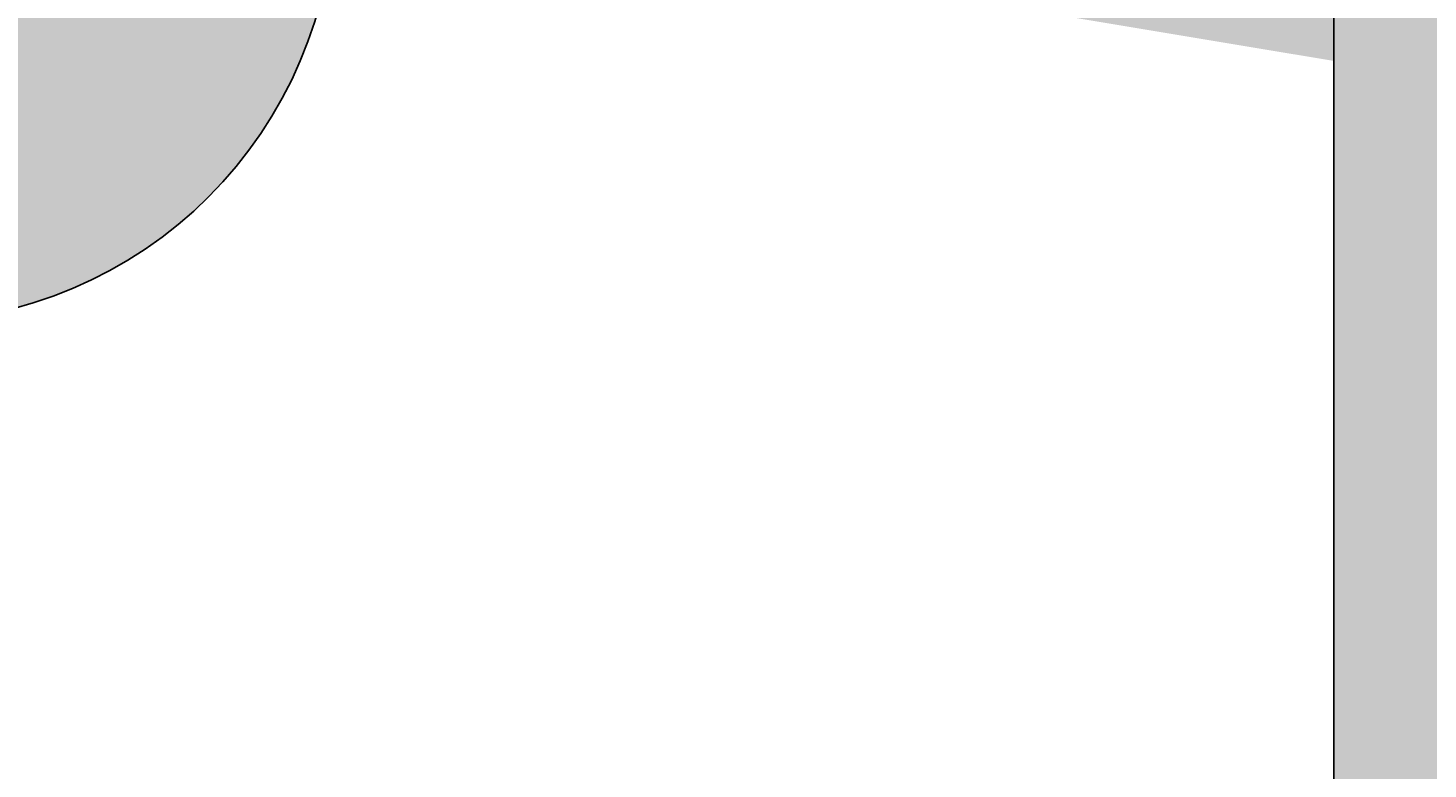
# Model space of a CAD drawing. Units: millimetres. Extents: x -22994 to 29398, y -19990 to 20176.
# Tile 18 of 135: x 54 to 99, y 52 to 76. Entities that reach past the tile are written whole.
import ezdxf

# ---------------------------------------------------------------- set-up
doc = ezdxf.new("R2010")
doc.units = ezdxf.units.MM
doc.header["$MEASUREMENT"] = 0
for name, color, linetype, lineweight in [('M-DIMS', 2, 'Continuous', 18), ('M-EQPM', 7, 'Continuous', 25), ('M-EQPM-PATT', 7, 'Continuous', 18)]:
    doc.layers.add(name, color=color, linetype=linetype, lineweight=lineweight)
doc.styles.get("Standard").update_dxf_attribs({"font": 'arial.ttf'})
doc.dimstyles.get("Standard").update_dxf_attribs({"dimtxt": 0.18, "dimasz": 10000, "dimexe": 0.18, "dimexo": 0.0625, "dimgap": 0.09, "dimtad": 0, "dimtih": 1, "dimtoh": 1, "dimdec": 0, "dimzin": 0, "dimdsep": 46, "dimtxsty": 'Standard', "dimcen": 0.09, "dimadec": 0, "dimazin": 0, "dimtfac": 1, "dimtdec": 0, "dimtofl": 0, "dimtmove": 0, "dimatfit": 3, "dimfxl": 1, "dimtolj": 1, "dimtzin": 0, "dimlwd": 30, "dimarcsym": 0})

# ---------------------------------------------------------------- blocks, each defined once
blk = doc.blocks.new('*D2')
at = {"layer": 'Defpoints', "color": 0, "transparency": 16777216}
for p in [(6.677, 10.271), (290.852, 10.271), (290.852, -5.079)]:
    blk.add_point(p, dxfattribs=at)
at = {"layer": 'M-DIMS', "color": 0, "lineweight": -2, "transparency": 16777216}
for p, q in [((6.677, 10.209), (6.677, -5.259)), ((290.852, 10.209), (290.852, -5.259))]:
    blk.add_line(p, q, dxfattribs=at)
at = {"layer": 'M-DIMS', "color": 0, "lineweight": 30, "transparency": 16777216}
for p, q in [((-9993.323, -5.079), (-19993.323, -5.079)), ((10290.852, -5.079), (20290.852, -5.079))]:
    blk.add_line(p, q, dxfattribs=at)
at = {"layer": 'M-DIMS', "color": 0, "transparency": 16777216}
for points in [[(-9993.323, 1661.588), (-9993.323, -1671.745), (6.677, -5.079)], [(10290.852, 1661.588), (10290.852, -1671.745), (290.852, -5.079)]]:
    blk.add_solid(points, dxfattribs=at)
at = {"layer": 'M-DIMS', "color": 0, "transparency": 16777216, "insert": (148.765, -5.079), "char_height": 0.18, "attachment_point": 5}
blk.add_mtext('\\A1;284.2', dxfattribs=at)
blk = doc.blocks.new('*D3')
at = {"layer": 'Defpoints', "color": 0, "transparency": 16777216}
for p in [(110.265, 204.165), (110.265, 176.366), (95.833, 127.967)]:
    blk.add_point(p, dxfattribs=at)
at = {"layer": 'M-DIMS', "color": 0, "lineweight": 30, "transparency": 16777216}
for p, q in [((-9904.167, 204.165), (-19904.167, 204.165)), ((10110.265, 204.165), (20110.265, 204.165))]:
    blk.add_line(p, q, dxfattribs=at)
at = {"layer": 'M-DIMS', "color": 0, "lineweight": -2, "transparency": 16777216}
for p, q in [((95.833, 128.03), (95.833, 204.345)), ((110.265, 176.429), (110.265, 204.345))]:
    blk.add_line(p, q, dxfattribs=at)
at = {"layer": 'M-DIMS', "color": 0, "transparency": 16777216}
for points in [[(-9904.167, 1870.832), (-9904.167, -1462.501), (95.833, 204.165)], [(10110.265, 1870.832), (10110.265, -1462.501), (110.265, 204.165)]]:
    blk.add_solid(points, dxfattribs=at)
at = {"layer": 'M-DIMS', "color": 0, "transparency": 16777216, "insert": (103.049, 204.165), "char_height": 0.18, "attachment_point": 5}
blk.add_mtext('\\A1;14.432', dxfattribs=at)
blk = doc.blocks.new('*D4')
at = {"layer": 'Defpoints', "color": 0, "transparency": 16777216}
for p in [(116.265, 204.165), (110.265, 176.366), (116.265, 176.366)]:
    blk.add_point(p, dxfattribs=at)
at = {"layer": 'M-DIMS', "color": 0, "lineweight": 30, "transparency": 16777216}
for p, q in [((-9889.735, 204.165), (-19889.735, 204.165)), ((10116.265, 204.165), (20116.265, 204.165))]:
    blk.add_line(p, q, dxfattribs=at)
at = {"layer": 'M-DIMS', "color": 0, "lineweight": -2, "transparency": 16777216}
for p, q in [((110.265, 176.429), (110.265, 204.345)), ((116.265, 176.429), (116.265, 204.345))]:
    blk.add_line(p, q, dxfattribs=at)
at = {"layer": 'M-DIMS', "color": 0, "transparency": 16777216}
for points in [[(-9889.735, 1870.832), (-9889.735, -1462.501), (110.265, 204.165)], [(10116.265, 1870.832), (10116.265, -1462.501), (116.265, 204.165)]]:
    blk.add_solid(points, dxfattribs=at)
at = {"layer": 'M-DIMS', "color": 0, "transparency": 16777216, "insert": (113.265, 204.165), "char_height": 0.18, "attachment_point": 5}
blk.add_mtext('\\A1;6', dxfattribs=at)
blk = doc.blocks.new('*D5')
at = {"layer": 'Defpoints', "color": 0, "transparency": 16777216}
for p in [(181.265, 204.165), (116.265, 176.366), (181.265, 176.366)]:
    blk.add_point(p, dxfattribs=at)
at = {"layer": 'M-DIMS', "color": 0, "lineweight": 30, "transparency": 16777216}
for p, q in [((-9883.735, 204.165), (-19883.735, 204.165)), ((10181.265, 204.165), (20181.265, 204.165))]:
    blk.add_line(p, q, dxfattribs=at)
at = {"layer": 'M-DIMS', "color": 0, "lineweight": -2, "transparency": 16777216}
for p, q in [((116.265, 176.429), (116.265, 204.345)), ((181.265, 176.429), (181.265, 204.345))]:
    blk.add_line(p, q, dxfattribs=at)
at = {"layer": 'M-DIMS', "color": 0, "transparency": 16777216}
for points in [[(-9883.735, 1870.832), (-9883.735, -1462.501), (116.265, 204.165)], [(10181.265, 1870.832), (10181.265, -1462.501), (181.265, 204.165)]]:
    blk.add_solid(points, dxfattribs=at)
at = {"layer": 'M-DIMS', "color": 0, "transparency": 16777216, "insert": (148.765, 204.165), "char_height": 0.18, "attachment_point": 5}
blk.add_mtext('\\A1;65', dxfattribs=at)
blk = doc.blocks.new('*D6')
at = {"layer": 'Defpoints', "color": 0, "transparency": 16777216}
for p in [(187.265, 204.165), (181.265, 176.366), (187.265, 176.366)]:
    blk.add_point(p, dxfattribs=at)
at = {"layer": 'M-DIMS', "color": 0, "lineweight": 30, "transparency": 16777216}
for p, q in [((-9818.735, 204.165), (-19818.735, 204.165)), ((10187.265, 204.165), (20187.265, 204.165))]:
    blk.add_line(p, q, dxfattribs=at)
at = {"layer": 'M-DIMS', "color": 0, "lineweight": -2, "transparency": 16777216}
for p, q in [((181.265, 176.429), (181.265, 204.345)), ((187.265, 176.429), (187.265, 204.345))]:
    blk.add_line(p, q, dxfattribs=at)
at = {"layer": 'M-DIMS', "color": 0, "transparency": 16777216}
for points in [[(-9818.735, 1870.832), (-9818.735, -1462.501), (181.265, 204.165)], [(10187.265, 1870.832), (10187.265, -1462.501), (187.265, 204.165)]]:
    blk.add_solid(points, dxfattribs=at)
at = {"layer": 'M-DIMS', "color": 0, "transparency": 16777216, "insert": (184.265, 204.165), "char_height": 0.18, "attachment_point": 5}
blk.add_mtext('\\A1;6', dxfattribs=at)
blk = doc.blocks.new('*D7')
at = {"layer": 'Defpoints', "color": 0, "transparency": 16777216}
for p in [(201.697, 204.165), (187.265, 176.366), (201.697, 127.967)]:
    blk.add_point(p, dxfattribs=at)
at = {"layer": 'M-DIMS', "color": 0, "lineweight": 30, "transparency": 16777216}
for p, q in [((-9812.735, 204.165), (-19812.735, 204.165)), ((10201.697, 204.165), (20201.697, 204.165))]:
    blk.add_line(p, q, dxfattribs=at)
at = {"layer": 'M-DIMS', "color": 0, "lineweight": -2, "transparency": 16777216}
for p, q in [((187.265, 176.429), (187.265, 204.345)), ((201.697, 128.03), (201.697, 204.345))]:
    blk.add_line(p, q, dxfattribs=at)
at = {"layer": 'M-DIMS', "color": 0, "transparency": 16777216}
for points in [[(-9812.735, 1870.832), (-9812.735, -1462.501), (187.265, 204.165)], [(10201.697, 1870.832), (10201.697, -1462.501), (201.697, 204.165)]]:
    blk.add_solid(points, dxfattribs=at)
at = {"layer": 'M-DIMS', "color": 0, "transparency": 16777216, "insert": (194.481, 204.165), "char_height": 0.18, "attachment_point": 5}
blk.add_mtext('\\A1;14.432', dxfattribs=at)
blk = doc.blocks.new('*D8')
at = {"layer": 'Defpoints', "color": 0, "transparency": 16777216}
for p in [(227.648, 204.165), (227.648, 146.73), (201.697, 127.967)]:
    blk.add_point(p, dxfattribs=at)
at = {"layer": 'M-DIMS', "color": 0, "lineweight": 30, "transparency": 16777216}
for p, q in [((-9798.303, 204.165), (-19798.303, 204.165)), ((10227.648, 204.165), (20227.648, 204.165))]:
    blk.add_line(p, q, dxfattribs=at)
at = {"layer": 'M-DIMS', "color": 0, "lineweight": -2, "transparency": 16777216}
for p, q in [((201.697, 128.03), (201.697, 204.345)), ((227.648, 146.792), (227.648, 204.345))]:
    blk.add_line(p, q, dxfattribs=at)
at = {"layer": 'M-DIMS', "color": 0, "transparency": 16777216}
for points in [[(-9798.303, 1870.832), (-9798.303, -1462.501), (201.697, 204.165)], [(10227.648, 1870.832), (10227.648, -1462.501), (227.648, 204.165)]]:
    blk.add_solid(points, dxfattribs=at)
at = {"layer": 'M-DIMS', "color": 0, "transparency": 16777216, "insert": (214.673, 204.165), "char_height": 0.18, "attachment_point": 5}
blk.add_mtext('\\A1;25.95', dxfattribs=at)
blk = doc.blocks.new('*D9')
at = {"layer": 'Defpoints', "color": 0, "transparency": 16777216}
for p in [(187.265, 176.366), (306.202, 176.366), (290.852, 10.271)]:
    blk.add_point(p, dxfattribs=at)
at = {"layer": 'M-DIMS', "color": 0, "lineweight": 30, "transparency": 16777216}
for p, q in [((306.202, 10176.366), (306.202, 20176.366)), ((306.202, -9989.729), (306.202, -19989.729))]:
    blk.add_line(p, q, dxfattribs=at)
at = {"layer": 'M-DIMS', "color": 0, "lineweight": -2, "transparency": 16777216}
for p, q in [((187.327, 176.366), (306.382, 176.366)), ((290.915, 10.271), (306.382, 10.271))]:
    blk.add_line(p, q, dxfattribs=at)
at = {"layer": 'M-DIMS', "color": 0, "transparency": 16777216}
for points in [[(-1360.465, 10176.366), (1972.869, 10176.366), (306.202, 176.366)], [(-1360.465, -9989.729), (1972.869, -9989.729), (306.202, 10.271)]]:
    blk.add_solid(points, dxfattribs=at)
at = {"layer": 'M-DIMS', "color": 0, "transparency": 16777216, "insert": (306.202, 93.319), "char_height": 0.18, "attachment_point": 5}
blk.add_mtext('\\A1;166.1', dxfattribs=at)
blk = doc.blocks.new('*D10')
at = {"layer": 'Defpoints', "color": 0, "transparency": 16777216}
for p in [(125.65, 136.071), (133.346, 136.071), (133.346, -5.079)]:
    blk.add_point(p, dxfattribs=at)
at = {"layer": 'M-DIMS', "color": 0, "lineweight": -2, "transparency": 16777216}
for p, q in [((125.65, 136.009), (125.65, -5.259)), ((133.346, 136.009), (133.346, -5.259))]:
    blk.add_line(p, q, dxfattribs=at)
at = {"layer": 'M-DIMS', "color": 0, "lineweight": 30, "transparency": 16777216}
for p, q in [((-9874.35, -5.079), (-19874.35, -5.079)), ((10133.346, -5.079), (20133.346, -5.079))]:
    blk.add_line(p, q, dxfattribs=at)
at = {"layer": 'M-DIMS', "color": 0, "transparency": 16777216}
for points in [[(-9874.35, 1661.588), (-9874.35, -1671.745), (125.65, -5.079)], [(10133.346, 1661.588), (10133.346, -1671.745), (133.346, -5.079)]]:
    blk.add_solid(points, dxfattribs=at)
at = {"layer": 'M-DIMS', "color": 0, "transparency": 16777216, "insert": (129.498, -5.079), "char_height": 0.18, "attachment_point": 5}
blk.add_mtext('\\A1;7.696', dxfattribs=at)
blk = doc.blocks.new('*D11')
at = {"layer": 'Defpoints', "color": 0, "transparency": 16777216}
for p in [(133.346, 136.071), (135.65, 136.071), (135.65, -5.079)]:
    blk.add_point(p, dxfattribs=at)
at = {"layer": 'M-DIMS', "color": 0, "lineweight": -2, "transparency": 16777216}
for p, q in [((133.346, 136.009), (133.346, -5.259)), ((135.65, 136.009), (135.65, -5.259))]:
    blk.add_line(p, q, dxfattribs=at)
at = {"layer": 'M-DIMS', "color": 0, "lineweight": 30, "transparency": 16777216}
for p, q in [((-9866.654, -5.079), (-19866.654, -5.079)), ((10135.65, -5.079), (20135.65, -5.079))]:
    blk.add_line(p, q, dxfattribs=at)
at = {"layer": 'M-DIMS', "color": 0, "transparency": 16777216}
for points in [[(-9866.654, 1661.588), (-9866.654, -1671.745), (133.346, -5.079)], [(10135.65, 1661.588), (10135.65, -1671.745), (135.65, -5.079)]]:
    blk.add_solid(points, dxfattribs=at)
at = {"layer": 'M-DIMS', "color": 0, "transparency": 16777216, "insert": (134.498, -5.079), "char_height": 0.18, "attachment_point": 5}
blk.add_mtext('\\A1;2.304', dxfattribs=at)
blk = doc.blocks.new('*D12')
at = {"layer": 'Defpoints', "color": 0, "transparency": 16777216}
for p in [(135.65, 136.071), (145.65, 136.071), (145.65, -5.079)]:
    blk.add_point(p, dxfattribs=at)
at = {"layer": 'M-DIMS', "color": 0, "lineweight": -2, "transparency": 16777216}
for p, q in [((135.65, 136.009), (135.65, -5.259)), ((145.65, 136.009), (145.65, -5.259))]:
    blk.add_line(p, q, dxfattribs=at)
at = {"layer": 'M-DIMS', "color": 0, "lineweight": 30, "transparency": 16777216}
for p, q in [((-9864.35, -5.079), (-19864.35, -5.079)), ((10145.65, -5.079), (20145.65, -5.079))]:
    blk.add_line(p, q, dxfattribs=at)
at = {"layer": 'M-DIMS', "color": 0, "transparency": 16777216}
for points in [[(-9864.35, 1661.588), (-9864.35, -1671.745), (135.65, -5.079)], [(10145.65, 1661.588), (10145.65, -1671.745), (145.65, -5.079)]]:
    blk.add_solid(points, dxfattribs=at)
at = {"layer": 'M-DIMS', "color": 0, "transparency": 16777216, "insert": (140.65, -5.079), "char_height": 0.18, "attachment_point": 5}
blk.add_mtext('\\A1;10', dxfattribs=at)
blk = doc.blocks.new('*D13')
at = {"layer": 'Defpoints', "color": 0, "transparency": 16777216}
for p in [(145.65, 136.071), (155.65, 136.071), (155.65, -5.079)]:
    blk.add_point(p, dxfattribs=at)
at = {"layer": 'M-DIMS', "color": 0, "lineweight": -2, "transparency": 16777216}
for p, q in [((145.65, 136.009), (145.65, -5.259)), ((155.65, 136.009), (155.65, -5.259))]:
    blk.add_line(p, q, dxfattribs=at)
at = {"layer": 'M-DIMS', "color": 0, "lineweight": 30, "transparency": 16777216}
for p, q in [((-9854.35, -5.079), (-19854.35, -5.079)), ((10155.65, -5.079), (20155.65, -5.079))]:
    blk.add_line(p, q, dxfattribs=at)
at = {"layer": 'M-DIMS', "color": 0, "transparency": 16777216}
for points in [[(-9854.35, 1661.588), (-9854.35, -1671.745), (145.65, -5.079)], [(10155.65, 1661.588), (10155.65, -1671.745), (155.65, -5.079)]]:
    blk.add_solid(points, dxfattribs=at)
at = {"layer": 'M-DIMS', "color": 0, "transparency": 16777216, "insert": (150.65, -5.079), "char_height": 0.18, "attachment_point": 5}
blk.add_mtext('\\A1;10', dxfattribs=at)
blk = doc.blocks.new('*D14')
at = {"layer": 'Defpoints', "color": 0, "transparency": 16777216}
for p in [(155.65, 136.071), (165.65, 136.071), (165.65, -5.079)]:
    blk.add_point(p, dxfattribs=at)
at = {"layer": 'M-DIMS', "color": 0, "lineweight": -2, "transparency": 16777216}
for p, q in [((155.65, 136.009), (155.65, -5.259)), ((165.65, 136.009), (165.65, -5.259))]:
    blk.add_line(p, q, dxfattribs=at)
at = {"layer": 'M-DIMS', "color": 0, "lineweight": 30, "transparency": 16777216}
for p, q in [((-9844.35, -5.079), (-19844.35, -5.079)), ((10165.65, -5.079), (20165.65, -5.079))]:
    blk.add_line(p, q, dxfattribs=at)
at = {"layer": 'M-DIMS', "color": 0, "transparency": 16777216}
for points in [[(-9844.35, 1661.588), (-9844.35, -1671.745), (155.65, -5.079)], [(10165.65, 1661.588), (10165.65, -1671.745), (165.65, -5.079)]]:
    blk.add_solid(points, dxfattribs=at)
at = {"layer": 'M-DIMS', "color": 0, "transparency": 16777216, "insert": (160.65, -5.079), "char_height": 0.18, "attachment_point": 5}
blk.add_mtext('\\A1;10', dxfattribs=at)
blk = doc.blocks.new('*D15')
at = {"layer": 'Defpoints', "color": 0, "transparency": 16777216}
for p in [(173.346, 154.788), (173.346, 136.071), (306.202, 136.071)]:
    blk.add_point(p, dxfattribs=at)
at = {"layer": 'M-DIMS', "color": 0, "lineweight": 30, "transparency": 16777216}
for p, q in [((306.202, 10154.788), (306.202, 20154.788)), ((306.202, -9863.929), (306.202, -19863.929))]:
    blk.add_line(p, q, dxfattribs=at)
at = {"layer": 'M-DIMS', "color": 0, "lineweight": -2, "transparency": 16777216}
for p, q in [((173.408, 154.788), (306.382, 154.788)), ((173.408, 136.071), (306.382, 136.071))]:
    blk.add_line(p, q, dxfattribs=at)
at = {"layer": 'M-DIMS', "color": 0, "transparency": 16777216}
for points in [[(-1360.465, 10154.788), (1972.869, 10154.788), (306.202, 154.788)], [(-1360.465, -9863.929), (1972.869, -9863.929), (306.202, 136.071)]]:
    blk.add_solid(points, dxfattribs=at)
at = {"layer": 'M-DIMS', "color": 0, "transparency": 16777216, "insert": (306.202, 145.43), "char_height": 0.18, "attachment_point": 5}
blk.add_mtext('\\A1;18.717', dxfattribs=at)
blk = doc.blocks.new('*D16')
at = {"layer": 'Defpoints', "color": 0, "transparency": 16777216}
for p in [(120.17, 204.165), (110.466, 48.035), (120.17, 48.035)]:
    blk.add_point(p, dxfattribs=at)
at = {"layer": 'M-DIMS', "color": 0, "lineweight": 30, "transparency": 16777216}
for p, q in [((-9889.534, 204.165), (-19889.534, 204.165)), ((10120.17, 204.165), (20120.17, 204.165))]:
    blk.add_line(p, q, dxfattribs=at)
at = {"layer": 'M-DIMS', "color": 0, "lineweight": -2, "transparency": 16777216}
for p, q in [((110.466, 48.097), (110.466, 204.345)), ((120.17, 48.097), (120.17, 204.345))]:
    blk.add_line(p, q, dxfattribs=at)
at = {"layer": 'M-DIMS', "color": 0, "transparency": 16777216}
for points in [[(-9889.534, 1870.832), (-9889.534, -1462.501), (110.466, 204.165)], [(10120.17, 1870.832), (10120.17, -1462.501), (120.17, 204.165)]]:
    blk.add_solid(points, dxfattribs=at)
at = {"layer": 'M-DIMS', "color": 0, "transparency": 16777216, "insert": (115.318, 204.165), "char_height": 0.18, "attachment_point": 5}
blk.add_mtext('\\A1;9.704', dxfattribs=at)
blk = doc.blocks.new('*D17')
at = {"layer": 'Defpoints', "color": 0, "transparency": 16777216}
for p in [(126.17, 204.165), (120.17, 48.035), (126.17, 48.035)]:
    blk.add_point(p, dxfattribs=at)
at = {"layer": 'M-DIMS', "color": 0, "lineweight": 30, "transparency": 16777216}
for p, q in [((-9879.83, 204.165), (-19879.83, 204.165)), ((10126.17, 204.165), (20126.17, 204.165))]:
    blk.add_line(p, q, dxfattribs=at)
at = {"layer": 'M-DIMS', "color": 0, "lineweight": -2, "transparency": 16777216}
for p, q in [((120.17, 48.097), (120.17, 204.345)), ((126.17, 48.097), (126.17, 204.345))]:
    blk.add_line(p, q, dxfattribs=at)
at = {"layer": 'M-DIMS', "color": 0, "transparency": 16777216}
for points in [[(-9879.83, 1870.832), (-9879.83, -1462.501), (120.17, 204.165)], [(10126.17, 1870.832), (10126.17, -1462.501), (126.17, 204.165)]]:
    blk.add_solid(points, dxfattribs=at)
at = {"layer": 'M-DIMS', "color": 0, "transparency": 16777216, "insert": (123.17, 204.165), "char_height": 0.18, "attachment_point": 5}
blk.add_mtext('\\A1;6', dxfattribs=at)
blk = doc.blocks.new('*D18')
at = {"layer": 'Defpoints', "color": 0, "transparency": 16777216}
for p in [(132.17, 204.165), (126.17, 48.035), (132.17, 48.035)]:
    blk.add_point(p, dxfattribs=at)
at = {"layer": 'M-DIMS', "color": 0, "lineweight": 30, "transparency": 16777216}
for p, q in [((-9873.83, 204.165), (-19873.83, 204.165)), ((10132.17, 204.165), (20132.17, 204.165))]:
    blk.add_line(p, q, dxfattribs=at)
at = {"layer": 'M-DIMS', "color": 0, "lineweight": -2, "transparency": 16777216}
for p, q in [((126.17, 48.097), (126.17, 204.345)), ((132.17, 48.097), (132.17, 204.345))]:
    blk.add_line(p, q, dxfattribs=at)
at = {"layer": 'M-DIMS', "color": 0, "transparency": 16777216}
for points in [[(-9873.83, 1870.832), (-9873.83, -1462.501), (126.17, 204.165)], [(10132.17, 1870.832), (10132.17, -1462.501), (132.17, 204.165)]]:
    blk.add_solid(points, dxfattribs=at)
at = {"layer": 'M-DIMS', "color": 0, "transparency": 16777216, "insert": (129.17, 204.165), "char_height": 0.18, "attachment_point": 5}
blk.add_mtext('\\A1;6', dxfattribs=at)
blk = doc.blocks.new('*D19')
at = {"layer": 'Defpoints', "color": 0, "transparency": 16777216}
for p in [(138.17, 204.165), (132.17, 48.035), (138.17, 48.035)]:
    blk.add_point(p, dxfattribs=at)
at = {"layer": 'M-DIMS', "color": 0, "lineweight": 30, "transparency": 16777216}
for p, q in [((-9867.83, 204.165), (-19867.83, 204.165)), ((10138.17, 204.165), (20138.17, 204.165))]:
    blk.add_line(p, q, dxfattribs=at)
at = {"layer": 'M-DIMS', "color": 0, "lineweight": -2, "transparency": 16777216}
for p, q in [((132.17, 48.097), (132.17, 204.345)), ((138.17, 48.097), (138.17, 204.345))]:
    blk.add_line(p, q, dxfattribs=at)
at = {"layer": 'M-DIMS', "color": 0, "transparency": 16777216}
for points in [[(-9867.83, 1870.832), (-9867.83, -1462.501), (132.17, 204.165)], [(10138.17, 1870.832), (10138.17, -1462.501), (138.17, 204.165)]]:
    blk.add_solid(points, dxfattribs=at)
at = {"layer": 'M-DIMS', "color": 0, "transparency": 16777216, "insert": (135.17, 204.165), "char_height": 0.18, "attachment_point": 5}
blk.add_mtext('\\A1;6', dxfattribs=at)
blk = doc.blocks.new('*D20')
at = {"layer": 'Defpoints', "color": 0, "transparency": 16777216}
for p in [(144.17, 204.165), (138.17, 48.035), (144.17, 48.035)]:
    blk.add_point(p, dxfattribs=at)
at = {"layer": 'M-DIMS', "color": 0, "lineweight": 30, "transparency": 16777216}
for p, q in [((-9861.83, 204.165), (-19861.83, 204.165)), ((10144.17, 204.165), (20144.17, 204.165))]:
    blk.add_line(p, q, dxfattribs=at)
at = {"layer": 'M-DIMS', "color": 0, "lineweight": -2, "transparency": 16777216}
for p, q in [((138.17, 48.097), (138.17, 204.345)), ((144.17, 48.097), (144.17, 204.345))]:
    blk.add_line(p, q, dxfattribs=at)
at = {"layer": 'M-DIMS', "color": 0, "transparency": 16777216}
for points in [[(-9861.83, 1870.832), (-9861.83, -1462.501), (138.17, 204.165)], [(10144.17, 1870.832), (10144.17, -1462.501), (144.17, 204.165)]]:
    blk.add_solid(points, dxfattribs=at)
at = {"layer": 'M-DIMS', "color": 0, "transparency": 16777216, "insert": (141.17, 204.165), "char_height": 0.18, "attachment_point": 5}
blk.add_mtext('\\A1;6', dxfattribs=at)
blk = doc.blocks.new('*D21')
at = {"layer": 'Defpoints', "color": 0, "transparency": 16777216}
for p in [(149.116, 204.165), (144.17, 48.035), (149.116, 48.035)]:
    blk.add_point(p, dxfattribs=at)
at = {"layer": 'M-DIMS', "color": 0, "lineweight": 30, "transparency": 16777216}
for p, q in [((-9855.83, 204.165), (-19855.83, 204.165)), ((10149.116, 204.165), (20149.116, 204.165))]:
    blk.add_line(p, q, dxfattribs=at)
at = {"layer": 'M-DIMS', "color": 0, "lineweight": -2, "transparency": 16777216}
for p, q in [((144.17, 48.097), (144.17, 204.345)), ((149.116, 48.097), (149.116, 204.345))]:
    blk.add_line(p, q, dxfattribs=at)
at = {"layer": 'M-DIMS', "color": 0, "transparency": 16777216}
for points in [[(-9855.83, 1870.832), (-9855.83, -1462.501), (144.17, 204.165)], [(10149.116, 1870.832), (10149.116, -1462.501), (149.116, 204.165)]]:
    blk.add_solid(points, dxfattribs=at)
at = {"layer": 'M-DIMS', "color": 0, "transparency": 16777216, "insert": (146.643, 204.165), "char_height": 0.18, "attachment_point": 5}
blk.add_mtext('\\A1;4.945', dxfattribs=at)
blk = doc.blocks.new('*D22')
at = {"layer": 'Defpoints', "color": 0, "transparency": 16777216}
for p in [(149.116, 30.99), (155.116, 30.99), (155.116, -5.079)]:
    blk.add_point(p, dxfattribs=at)
at = {"layer": 'M-DIMS', "color": 0, "lineweight": -2, "transparency": 16777216}
for p, q in [((149.116, 30.927), (149.116, -5.259)), ((155.116, 30.927), (155.116, -5.259))]:
    blk.add_line(p, q, dxfattribs=at)
at = {"layer": 'M-DIMS', "color": 0, "lineweight": 30, "transparency": 16777216}
for p, q in [((-9850.884, -5.079), (-19850.884, -5.079)), ((10155.116, -5.079), (20155.116, -5.079))]:
    blk.add_line(p, q, dxfattribs=at)
at = {"layer": 'M-DIMS', "color": 0, "transparency": 16777216}
for points in [[(-9850.884, 1661.588), (-9850.884, -1671.745), (149.116, -5.079)], [(10155.116, 1661.588), (10155.116, -1671.745), (155.116, -5.079)]]:
    blk.add_solid(points, dxfattribs=at)
at = {"layer": 'M-DIMS', "color": 0, "transparency": 16777216, "insert": (152.116, -5.079), "char_height": 0.18, "attachment_point": 5}
blk.add_mtext('\\A1;6', dxfattribs=at)
blk = doc.blocks.new('*D23')
at = {"layer": 'Defpoints', "color": 0, "transparency": 16777216}
for p in [(155.116, 30.99), (161.116, 30.99), (161.116, -5.079)]:
    blk.add_point(p, dxfattribs=at)
at = {"layer": 'M-DIMS', "color": 0, "lineweight": -2, "transparency": 16777216}
for p, q in [((155.116, 30.927), (155.116, -5.259)), ((161.116, 30.927), (161.116, -5.259))]:
    blk.add_line(p, q, dxfattribs=at)
at = {"layer": 'M-DIMS', "color": 0, "lineweight": 30, "transparency": 16777216}
for p, q in [((-9844.884, -5.079), (-19844.884, -5.079)), ((10161.116, -5.079), (20161.116, -5.079))]:
    blk.add_line(p, q, dxfattribs=at)
at = {"layer": 'M-DIMS', "color": 0, "transparency": 16777216}
for points in [[(-9844.884, 1661.588), (-9844.884, -1671.745), (155.116, -5.079)], [(10161.116, 1661.588), (10161.116, -1671.745), (161.116, -5.079)]]:
    blk.add_solid(points, dxfattribs=at)
at = {"layer": 'M-DIMS', "color": 0, "transparency": 16777216, "insert": (158.116, -5.079), "char_height": 0.18, "attachment_point": 5}
blk.add_mtext('\\A1;6', dxfattribs=at)
blk = doc.blocks.new('*D24')
at = {"layer": 'Defpoints', "color": 0, "transparency": 16777216}
for p in [(161.116, 30.99), (166.439, 30.99), (166.439, -5.079)]:
    blk.add_point(p, dxfattribs=at)
at = {"layer": 'M-DIMS', "color": 0, "lineweight": -2, "transparency": 16777216}
for p, q in [((161.116, 30.927), (161.116, -5.259)), ((166.439, 30.927), (166.439, -5.259))]:
    blk.add_line(p, q, dxfattribs=at)
at = {"layer": 'M-DIMS', "color": 0, "lineweight": 30, "transparency": 16777216}
for p, q in [((-9838.884, -5.079), (-19838.884, -5.079)), ((10166.439, -5.079), (20166.439, -5.079))]:
    blk.add_line(p, q, dxfattribs=at)
at = {"layer": 'M-DIMS', "color": 0, "transparency": 16777216}
for points in [[(-9838.884, 1661.588), (-9838.884, -1671.745), (161.116, -5.079)], [(10166.439, 1661.588), (10166.439, -1671.745), (166.439, -5.079)]]:
    blk.add_solid(points, dxfattribs=at)
at = {"layer": 'M-DIMS', "color": 0, "transparency": 16777216, "insert": (163.777, -5.079), "char_height": 0.18, "attachment_point": 5}
blk.add_mtext('\\A1;5.323', dxfattribs=at)
blk = doc.blocks.new('*D25')
at = {"layer": 'Defpoints', "color": 0, "transparency": 16777216}
for p in [(166.439, 30.99), (172.439, 30.99), (172.439, -5.079)]:
    blk.add_point(p, dxfattribs=at)
at = {"layer": 'M-DIMS', "color": 0, "lineweight": -2, "transparency": 16777216}
for p, q in [((166.439, 30.927), (166.439, -5.259)), ((172.439, 30.927), (172.439, -5.259))]:
    blk.add_line(p, q, dxfattribs=at)
at = {"layer": 'M-DIMS', "color": 0, "lineweight": 30, "transparency": 16777216}
for p, q in [((-9833.561, -5.079), (-19833.561, -5.079)), ((10172.439, -5.079), (20172.439, -5.079))]:
    blk.add_line(p, q, dxfattribs=at)
at = {"layer": 'M-DIMS', "color": 0, "transparency": 16777216}
for points in [[(-9833.561, 1661.588), (-9833.561, -1671.745), (166.439, -5.079)], [(10172.439, 1661.588), (10172.439, -1671.745), (172.439, -5.079)]]:
    blk.add_solid(points, dxfattribs=at)
at = {"layer": 'M-DIMS', "color": 0, "transparency": 16777216, "insert": (169.439, -5.079), "char_height": 0.18, "attachment_point": 5}
blk.add_mtext('\\A1;6', dxfattribs=at)
blk = doc.blocks.new('*D26')
at = {"layer": 'Defpoints', "color": 0, "transparency": 16777216}
for p in [(172.439, 30.99), (178.439, 30.99), (178.439, -5.079)]:
    blk.add_point(p, dxfattribs=at)
at = {"layer": 'M-DIMS', "color": 0, "lineweight": -2, "transparency": 16777216}
for p, q in [((172.439, 30.927), (172.439, -5.259)), ((178.439, 30.927), (178.439, -5.259))]:
    blk.add_line(p, q, dxfattribs=at)
at = {"layer": 'M-DIMS', "color": 0, "lineweight": 30, "transparency": 16777216}
for p, q in [((-9827.561, -5.079), (-19827.561, -5.079)), ((10178.439, -5.079), (20178.439, -5.079))]:
    blk.add_line(p, q, dxfattribs=at)
at = {"layer": 'M-DIMS', "color": 0, "transparency": 16777216}
for points in [[(-9827.561, 1661.588), (-9827.561, -1671.745), (172.439, -5.079)], [(10178.439, 1661.588), (10178.439, -1671.745), (178.439, -5.079)]]:
    blk.add_solid(points, dxfattribs=at)
at = {"layer": 'M-DIMS', "color": 0, "transparency": 16777216, "insert": (175.439, -5.079), "char_height": 0.18, "attachment_point": 5}
blk.add_mtext('\\A1;6', dxfattribs=at)
blk = doc.blocks.new('*D27')
at = {"layer": 'Defpoints', "color": 0, "transparency": 16777216}
for p in [(178.439, 30.99), (188.117, 30.99), (188.117, -5.079)]:
    blk.add_point(p, dxfattribs=at)
at = {"layer": 'M-DIMS', "color": 0, "lineweight": -2, "transparency": 16777216}
for p, q in [((178.439, 30.927), (178.439, -5.259)), ((188.117, 30.927), (188.117, -5.259))]:
    blk.add_line(p, q, dxfattribs=at)
at = {"layer": 'M-DIMS', "color": 0, "lineweight": 30, "transparency": 16777216}
for p, q in [((-9821.561, -5.079), (-19821.561, -5.079)), ((10188.117, -5.079), (20188.117, -5.079))]:
    blk.add_line(p, q, dxfattribs=at)
at = {"layer": 'M-DIMS', "color": 0, "transparency": 16777216}
for points in [[(-9821.561, 1661.588), (-9821.561, -1671.745), (178.439, -5.079)], [(10188.117, 1661.588), (10188.117, -1671.745), (188.117, -5.079)]]:
    blk.add_solid(points, dxfattribs=at)
at = {"layer": 'M-DIMS', "color": 0, "transparency": 16777216, "insert": (183.278, -5.079), "char_height": 0.18, "attachment_point": 5}
blk.add_mtext('\\A1;9.679', dxfattribs=at)
blk = doc.blocks.new('*D28')
at = {"layer": 'Defpoints', "color": 0, "transparency": 16777216}
for p in [(188.117, 48.035), (306.202, 48.035), (188.117, 30.99)]:
    blk.add_point(p, dxfattribs=at)
at = {"layer": 'M-DIMS', "color": 0, "lineweight": 30, "transparency": 16777216}
for p, q in [((306.202, 10048.035), (306.202, 20048.035)), ((306.202, -9969.01), (306.202, -19969.01))]:
    blk.add_line(p, q, dxfattribs=at)
at = {"layer": 'M-DIMS', "color": 0, "lineweight": -2, "transparency": 16777216}
for p, q in [((188.18, 48.035), (306.382, 48.035)), ((188.18, 30.99), (306.382, 30.99))]:
    blk.add_line(p, q, dxfattribs=at)
at = {"layer": 'M-DIMS', "color": 0, "transparency": 16777216}
for points in [[(-1360.465, 10048.035), (1972.869, 10048.035), (306.202, 48.035)], [(-1360.465, -9969.01), (1972.869, -9969.01), (306.202, 30.99)]]:
    blk.add_solid(points, dxfattribs=at)
at = {"layer": 'M-DIMS', "color": 0, "transparency": 16777216, "insert": (306.202, 39.512), "char_height": 0.18, "attachment_point": 5}
blk.add_mtext('\\A1;17.045', dxfattribs=at)
blk = doc.blocks.new('*D29')
at = {"layer": 'Defpoints', "color": 0, "transparency": 16777216}
for p in [(36.801, 80.045), (64.03, 80.045)]:
    blk.add_point(p, dxfattribs=at)
at = {"layer": 'M-DIMS', "color": 0, "lineweight": -2, "transparency": 16777216}
for p, q in [((50.325, 80.045), (50.505, 80.045)), ((50.415, 79.955), (50.415, 80.135))]:
    blk.add_line(p, q, dxfattribs=at)
at = {"layer": 'M-DIMS', "color": 0, "lineweight": 30, "transparency": 16777216}
blk.add_line((20064.03, 80.03), (10064.03, 80.038), dxfattribs=at)
at = {"layer": 'M-DIMS', "color": 0, "transparency": 16777216}
blk.add_solid([(10064.031, 1746.704), (10064.028, -1586.629), (64.03, 80.045)], dxfattribs=at)
at = {"layer": 'M-DIMS', "color": 0, "transparency": 16777216, "insert": (20064.521, 80.03), "char_height": 0.18, "attachment_point": 5}
blk.add_mtext('\\A1;∅27.23', dxfattribs=at)
blk = doc.blocks.new('*D32')
at = {"layer": 'Defpoints', "color": 0, "transparency": 16777216}
for p in [(57.164, 118.614), (52.413, 113.093)]:
    blk.add_point(p, dxfattribs=at)
at = {"layer": 'M-DIMS', "color": 0, "lineweight": -2, "transparency": 16777216}
for p, q in [((57.074, 118.614), (57.254, 118.614)), ((57.164, 118.524), (57.164, 118.704))]:
    blk.add_line(p, q, dxfattribs=at)
at = {"layer": 'M-DIMS', "color": 0, "lineweight": 30, "transparency": 16777216}
for p, q in [((-12992.534, -15047.031), (-6470.06, -7466.969)), ((-22992.534, -15047.031), (-12992.534, -15047.031))]:
    blk.add_line(p, q, dxfattribs=at)
at = {"layer": 'M-DIMS', "color": 0, "transparency": 16777216}
blk.add_solid([(-7733.404, -6379.89), (-5206.717, -8554.048), (52.413, 113.093)], dxfattribs=at)
at = {"layer": 'M-DIMS', "color": 0, "transparency": 16777216, "insert": (-22993.208, -15047.031), "char_height": 0.18, "attachment_point": 5}
blk.add_mtext('\\A1;2X R7.284', dxfattribs=at)
blk = doc.blocks.new('*D36')
at = {"layer": 'Defpoints', "color": 0, "transparency": 16777216}
for p in [(46.39, 31.303), (46.387, 26.593)]:
    blk.add_point(p, dxfattribs=at)
at = {"layer": 'M-DIMS', "color": 0, "lineweight": 30, "transparency": 16777216}
for p, q in [((57.15, 20031.301), (51.77, 10031.302)), ((10057.15, 20031.301), (57.15, 20031.301))]:
    blk.add_line(p, q, dxfattribs=at)
at = {"layer": 'M-DIMS', "color": 0, "lineweight": -2, "transparency": 16777216}
for p, q in [((46.299, 28.948), (46.479, 28.948)), ((46.389, 28.858), (46.389, 29.038))]:
    blk.add_line(p, q, dxfattribs=at)
at = {"layer": 'M-DIMS', "color": 0, "transparency": 16777216}
blk.add_solid([(-1614.896, 10032.199), (1718.436, 10030.405), (46.39, 31.303)], dxfattribs=at)
at = {"layer": 'M-DIMS', "color": 0, "transparency": 16777216, "insert": (10057.554, 20031.301), "char_height": 0.18, "attachment_point": 5}
blk.add_mtext('\\A1;∅4.71', dxfattribs=at)
blk = doc.blocks.new('*D37')
at = {"layer": 'Defpoints', "color": 0, "transparency": 16777216}
for p in [(54.834, 118.615), (59.494, 118.614)]:
    blk.add_point(p, dxfattribs=at)
at = {"layer": 'M-DIMS', "color": 0, "lineweight": -2, "transparency": 16777216}
for p, q in [((57.074, 118.614), (57.254, 118.614)), ((57.164, 118.524), (57.164, 118.704))]:
    blk.add_line(p, q, dxfattribs=at)
at = {"layer": 'M-DIMS', "color": 0, "lineweight": 30, "transparency": 16777216}
blk.add_line((20059.493, 116.253), (10059.494, 117.434), dxfattribs=at)
at = {"layer": 'M-DIMS', "color": 0, "transparency": 16777216}
blk.add_solid([(10059.69, 1784.1), (10059.297, -1549.233), (59.494, 118.614)], dxfattribs=at)
at = {"layer": 'M-DIMS', "color": 0, "transparency": 16777216, "insert": (20059.985, 116.253), "char_height": 0.18, "attachment_point": 5}
blk.add_mtext('\\A1;∅4.659', dxfattribs=at)

msp = doc.modelspace()

# ---------------------------------------------------------------- hatches: boundary and pattern name
at = {"layer": 'M-EQPM-PATT'}
h = msp.add_hatch(color=256, dxfattribs=at)
h.set_gradient(color1=(205, 32, 39), color2=(205, 32, 39), tint=1)
h.paths.add_polyline_path([(116.2647, 150.3662), (116.2647, 170.3662), (116.2647, 176.3662), (110.2647, 176.3662), (110.2647, 152.0276), (95.8327, 127.967), (95.8327, 16.6063), (201.6967, 16.6063), (201.6967, 127.967), (187.2647, 152.0276), (187.2647, 176.3662), (181.2647, 176.3662), (181.2647, 170.3662), (181.2647, 150.3662), (195.6967, 126.3055), (195.6967, 22.6063), (101.8327, 22.6063), (101.8327, 126.3055)])
h.paths.add_polyline_path([(185.2208, 88.6347), (101.8327, 88.6347), (101.8327, 87.6347), (182.8066, 87.6347), (178.7313, 83.5594), (195.6967, 83.5594), (195.6967, 84.5594), (181.1455, 84.5594)], flags=17)
h.paths.add_polyline_path([(95.8327, 88.6347), (60.9779, 88.6347, -0.0228552), (61.7178, 87.6347), (95.8327, 87.6347)])
h.paths.add_polyline_path([(215.6212, 86.5189), (215.6212, 80.5999), (220.5095, 83.5594)])
h.paths.add_polyline_path([(215.6212, 84.5594), (201.6967, 84.5594), (201.6967, 83.5594), (215.6212, 83.5594)])
h.paths.add_polyline_path([(225.3978, 86.5189), (220.5095, 83.5594), (225.3978, 80.5999)])
h.paths.add_polyline_path([(231.6256, 84.5594), (225.3978, 84.5594), (225.3978, 83.5594), (231.6256, 83.5594)])
h = msp.add_hatch(color=256, dxfattribs=at)
h.set_gradient(color1=(0, 255, 255), color2=(41, 49, 137), tint=1, name='CYLINDER')
h.paths.add_polyline_path([(64.0296, 80.045, 1), (36.8006, 80.045, 1)])

# ---------------------------------------------------------------- linework, layer by layer
at = {"layer": 'M-EQPM'}
msp.add_lwpolyline([(110.2647, 176.3662), (110.2647, 152.0276), (95.8327, 127.967), (95.8327, 16.6063), (201.6967, 16.6063), (201.6967, 127.967), (187.2647, 152.0276), (187.2647, 176.3662)], close=True, dxfattribs=at)
msp.add_circle((50.4151, 80.045), 13.6145, dxfattribs=at)

# ---------------------------------------------------------------- dimensions: what is measured, and where the dimension line sits
at = {"layer": 'M-DIMS'}
for base, p1, p2, override, picture, middle in [((306.202, 176.3662), (290.852, 10.2713), (187.2647, 176.3662), {"dimdec": 1, "dimlfac": 1, "dimrnd": 0, "dimzin": 0, "dimdsep": 46, "dimlunit": 2}, '*D9', (306.202, 93.3187)), ((306.202, 136.0713), (173.3459, 154.788), (173.3459, 136.0713), {"dimdec": 3, "dimlfac": 1, "dimrnd": 0, "dimzin": 0, "dimdsep": 46, "dimlunit": 2}, '*D15', (306.202, 145.4297)), ((306.202, 48.0349), (188.1175, 30.9895), (188.1175, 48.0349), {"dimdec": 3, "dimlfac": 1, "dimrnd": 0, "dimzin": 0, "dimdsep": 46, "dimlunit": 2}, '*D28', (306.202, 39.5122))]:
    dim = msp.add_linear_dim(base=base, p1=p1, p2=p2, angle=90, dimstyle='Standard', override=override, dxfattribs=at)
    dim.commit()
    dim.dimension.update_dxf_attribs({"geometry": picture, "text_midpoint": middle})
dim = msp.add_diameter_dim_2p(p1=(46.3875, 26.5934), p2=(46.39, 31.3035), dimstyle='Standard', override={"dimdec": 2, "dimlfac": 1, "dimrnd": 0, "dimzin": 0, "dimdsep": 46, "dimlunit": 2}, dxfattribs=at)
dim.commit()
dim.dimension.update_dxf_attribs({"geometry": '*D36', "text_midpoint": (10057.5542, 20031.3006), "dimtype": 163})
for base, p1, p2, override, picture, middle in [((110.2647, 204.1654), (95.8327, 127.967), (110.2647, 176.3662), {"dimdec": 3, "dimlfac": 1, "dimrnd": 0, "dimzin": 0, "dimdsep": 46, "dimlunit": 2}, '*D3', (103.0487, 204.1654)), ((116.2647, 204.1654), (110.2647, 176.3662), (116.2647, 176.3662), {"dimdec": 0, "dimlfac": 1, "dimrnd": 0, "dimzin": 0, "dimdsep": 46, "dimlunit": 2}, '*D4', (113.2647, 204.1654)), ((120.1702, 204.1654), (110.4658, 48.0349), (120.1702, 48.0349), {"dimdec": 3, "dimlfac": 1, "dimrnd": 0, "dimzin": 0, "dimdsep": 46, "dimlunit": 2}, '*D16', (115.318, 204.1654)), ((181.2647, 204.1654), (116.2647, 176.3662), (181.2647, 176.3662), {"dimdec": 0, "dimlfac": 1, "dimrnd": 0, "dimzin": 0, "dimdsep": 46, "dimlunit": 2}, '*D5', (148.7647, 204.1654)), ((126.1702, 204.1654), (120.1702, 48.0349), (126.1702, 48.0349), {"dimdec": 0, "dimlfac": 1, "dimrnd": 0, "dimzin": 0, "dimdsep": 46, "dimlunit": 2}, '*D17', (123.1702, 204.1654)), ((132.1702, 204.1654), (126.1702, 48.0349), (132.1702, 48.0349), {"dimdec": 0, "dimlfac": 1, "dimrnd": 0, "dimzin": 0, "dimdsep": 46, "dimlunit": 2}, '*D18', (129.1702, 204.1654)), ((138.1702, 204.1654), (132.1702, 48.0349), (138.1702, 48.0349), {"dimdec": 0, "dimlfac": 1, "dimrnd": 0, "dimzin": 0, "dimdsep": 46, "dimlunit": 2}, '*D19', (135.1702, 204.1654)), ((144.1702, 204.1654), (138.1702, 48.0349), (144.1702, 48.0349), {"dimdec": 0, "dimlfac": 1, "dimrnd": 0, "dimzin": 0, "dimdsep": 46, "dimlunit": 2}, '*D20', (141.1702, 204.1654)), ((149.11567, 204.16539), (144.17023, 48.03494), (149.11567, 48.03494), {"dimdec": 3, "dimlfac": 1, "dimrnd": 0, "dimzin": 0, "dimdsep": 46, "dimlunit": 2}, '*D21', (146.64295, 204.16539)), ((187.2647, 204.1654), (181.2647, 176.3662), (187.2647, 176.3662), {"dimdec": 0, "dimlfac": 1, "dimrnd": 0, "dimzin": 0, "dimdsep": 46, "dimlunit": 2}, '*D6', (184.2647, 204.1654)), ((201.6967, 204.1654), (187.2647, 176.3662), (201.6967, 127.967), {"dimdec": 3, "dimlfac": 1, "dimrnd": 0, "dimzin": 0, "dimdsep": 46, "dimlunit": 2}, '*D7', (194.4807, 204.1654)), ((227.6485, 204.1654), (201.6967, 127.967), (227.6485, 146.7296), {"dimdec": 2, "dimlfac": 1, "dimrnd": 0, "dimzin": 0, "dimdsep": 46, "dimlunit": 2}, '*D8', (214.6726, 204.1654)), ((290.852, -5.0787), (6.6773, 10.2713), (290.852, 10.2713), {"dimdec": 1, "dimlfac": 1, "dimrnd": 0, "dimzin": 0, "dimdsep": 46, "dimlunit": 2}, '*D2', (148.7647, -5.0787)), ((133.3459, -5.0787), (125.6498, 136.0713), (133.3459, 136.0713), {"dimdec": 3, "dimlfac": 1, "dimrnd": 0, "dimzin": 0, "dimdsep": 46, "dimlunit": 2}, '*D10', (129.4978, -5.0787)), ((135.6498, -5.0787), (133.3459, 136.0713), (135.6498, 136.0713), {"dimdec": 3, "dimlfac": 1, "dimrnd": 0, "dimzin": 0, "dimdsep": 46, "dimlunit": 2}, '*D11', (134.4978, -5.0787)), ((145.6498, -5.0787), (135.6498, 136.0713), (145.6498, 136.0713), {"dimdec": 0, "dimlfac": 1, "dimrnd": 0, "dimzin": 0, "dimdsep": 46, "dimlunit": 2}, '*D12', (140.6498, -5.0787)), ((155.6498, -5.0787), (145.6498, 136.0713), (155.6498, 136.0713), {"dimdec": 0, "dimlfac": 1, "dimrnd": 0, "dimzin": 0, "dimdsep": 46, "dimlunit": 2}, '*D13', (150.6498, -5.0787)), ((155.1157, -5.0787), (149.1157, 30.9895), (155.1157, 30.9895), {"dimdec": 0, "dimlfac": 1, "dimrnd": 0, "dimzin": 0, "dimdsep": 46, "dimlunit": 2}, '*D22', (152.1157, -5.0787)), ((161.1157, -5.0787), (155.1157, 30.9895), (161.1157, 30.9895), {"dimdec": 0, "dimlfac": 1, "dimrnd": 0, "dimzin": 0, "dimdsep": 46, "dimlunit": 2}, '*D23', (158.1157, -5.0787)), ((165.6498, -5.0787), (155.6498, 136.0713), (165.6498, 136.0713), {"dimdec": 0, "dimlfac": 1, "dimrnd": 0, "dimzin": 0, "dimdsep": 46, "dimlunit": 2}, '*D14', (160.6498, -5.0787)), ((166.4387, -5.0787), (161.1157, 30.9895), (166.4387, 30.9895), {"dimdec": 3, "dimlfac": 1, "dimrnd": 0, "dimzin": 0, "dimdsep": 46, "dimlunit": 2}, '*D24', (163.7772, -5.0787)), ((172.4387, -5.0787), (166.4387, 30.9895), (172.4387, 30.9895), {"dimdec": 0, "dimlfac": 1, "dimrnd": 0, "dimzin": 0, "dimdsep": 46, "dimlunit": 2}, '*D25', (169.4387, -5.0787)), ((178.4387, -5.0787), (172.4387, 30.9895), (178.4387, 30.9895), {"dimdec": 0, "dimlfac": 1, "dimrnd": 0, "dimzin": 0, "dimdsep": 46, "dimlunit": 2}, '*D26', (175.4387, -5.0787)), ((188.1175, -5.0787), (178.4387, 30.9895), (188.1175, 30.9895), {"dimdec": 3, "dimlfac": 1, "dimrnd": 0, "dimzin": 0, "dimdsep": 46, "dimlunit": 2}, '*D27', (183.2781, -5.0787))]:
    dim = msp.add_linear_dim(base=base, p1=p1, p2=p2, dimstyle='Standard', override=override, dxfattribs=at)
    dim.commit()
    dim.dimension.update_dxf_attribs({"geometry": picture, "text_midpoint": middle})
for p1, p2, override, picture, middle in [((54.8343, 118.6145), (59.4936, 118.614), {"dimdec": 3, "dimlfac": 1, "dimrnd": 0, "dimzin": 0, "dimdsep": 46, "dimlunit": 2}, '*D37', (20059.4934, 116.2531)), ((36.8006, 80.045), (64.0296, 80.045), {"dimdec": 2, "dimlfac": 1, "dimrnd": 0, "dimzin": 0, "dimdsep": 46, "dimlunit": 2}, '*D29', (20064.0296, 80.0303))]:
    dim = msp.add_diameter_dim_2p(p1=p1, p2=p2, dimstyle='Standard', override=override, dxfattribs=at)
    dim.commit()
    dim.dimension.update_dxf_attribs({"geometry": picture, "text_midpoint": middle})
dim = msp.add_radius_dim(center=(57.1639, 118.6143), mpoint=(52.4129, 113.0929), text='2X <>', dimstyle='Standard', override={"dimdec": 3, "dimlfac": 1, "dimrnd": 0, "dimzin": 0, "dimdsep": 46, "dimlunit": 2}, dxfattribs=at)
dim.commit()
dim.dimension.update_dxf_attribs({"geometry": '*D32', "text_midpoint": (-22993.208, -15047.0314)})

doc.saveas('drawing.dxf')
